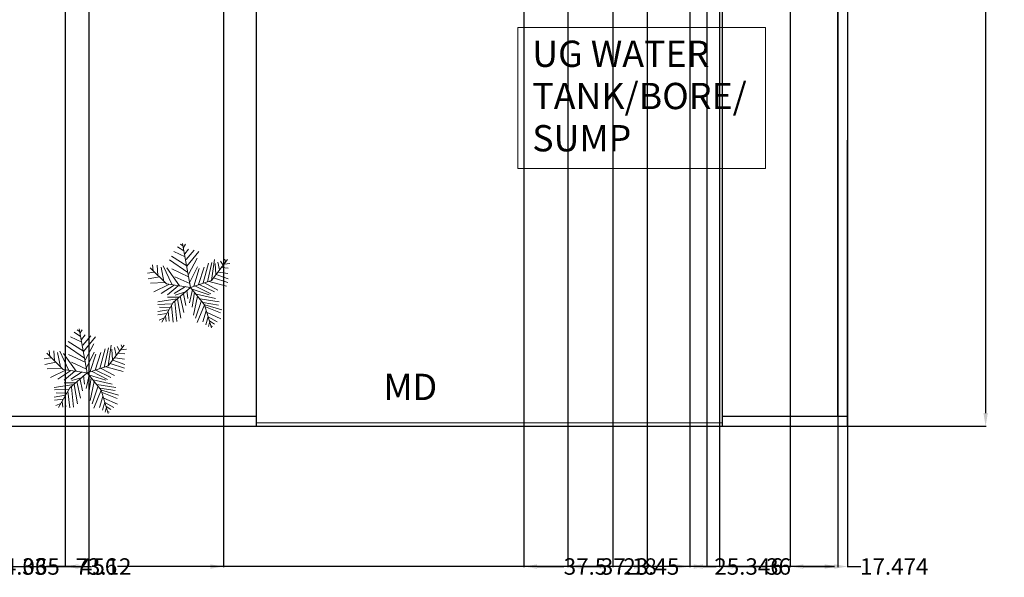
# Model space of a CAD drawing. Units: inches. Extents: x 460 to 1030, y -658 to 271.
# Tile 4 of 10: x 728 to 1028, y -658 to -488. Entities that reach past the tile are written whole.
import ezdxf

# ---------------------------------------------------------------- set-up
doc = ezdxf.new("R2010")
doc.units = ezdxf.units.IN
doc.header["$MEASUREMENT"] = 0
for name, color, linetype, lineweight in [('A-ANNO-DIMS', 2, 'Continuous', 18), ('A-ANNO-TEXT', 7, 'Continuous', 18), ('C-ANNO-TEXT', 7, 'Continuous', 18), ('C-PROP', 7, 'Continuous', 25), ('C-SITE-GATE', 3, 'Continuous', 18), ('C-UTIL', 8, 'Continuous', 18), ('L-PLNT', 94, 'Continuous', 13)]:
    doc.layers.add(name, color=color, linetype=linetype, lineweight=lineweight)
doc.styles.get("Standard").update_dxf_attribs({"font": 'arial.ttf'})
doc.dimstyles.get("Standard").update_dxf_attribs({"dimtxt": 5, "dimasz": 4, "dimexe": 0.18, "dimexo": 0.0625, "dimgap": 0.09, "dimtad": 0, "dimtih": 1, "dimtoh": 1, "dimdec": 1, "dimzin": 0, "dimdsep": 46, "dimlunit": 4, "dimtxsty": 'Standard', "dimcen": 0.09, "dimadec": 0, "dimazin": 0, "dimtfac": 1, "dimtdec": 1, "dimtofl": 0, "dimtmove": 0, "dimatfit": 3, "dimfxl": 1, "dimtolj": 1, "dimtzin": 0, "dimarcsym": 0})

# ---------------------------------------------------------------- blocks, each defined once
blk = doc.blocks.new('*U11')
for p, q in [((-221.9198, 1197.3052), (-433.5526, 1338.8594)), ((-258.7244, 1362.456), (-332.3336, 1421.4348)), ((0, 0), (-266.7, 1447.8)), ((-231.1146, 1315.2628), (-166.7002, 1421.4348)), ((-129.8956, 713.6638), (-626.7704, 1032.1544)), ((-185.1152, 1008.5578), (-553.1612, 1185.4942)), ((-194.31, 1102.9442), (-65.4812, 1256.284)), ((-148.3106, 914.1968), (118.5418, 1220.9018)), ((-129.8956, 701.8528), (265.7602, 1185.4942)), ((-1234.059, 536.7274), (-1252.4486, 737.2604)), ((-1105.2302, 725.4494), (-1077.6458, 395.1732)), ((-976.4268, 666.4706), (-884.4026, 194.6402)), ((-902.8176, 713.6638), (-617.5756, 100.2538)), ((-93.091, 489.5342), (-700.3796, 902.3858)), ((-74.7014, 418.7444), (219.7608, 961.39)), ((-28.6766, 171.0436), (228.9556, 678.2816)), ((256.5654, 88.4682), (449.7832, 666.4706)), ((412.9786, 147.447), (587.8068, 796.2392)), ((560.197, 182.8292), (698.2206, 819.8358)), ((685.8, 228.6), (1219.2, 914.4)), ((689.0258, 230.0224), (790.2448, 914.1968)), ((808.6344, 784.4282), (827.0494, 418.7444)), ((891.4384, 831.6214), (946.658, 572.1096)), ((983.4626, 867.0036), (1066.2666, 725.4494)), ((1029.462, 654.685), (1241.0948, 631.0884)), ((1112.2914, 760.8316), (1296.3144, 784.4282)), ((1121.4862, 925.9824), (1149.0706, 831.6214)), ((-1206.4492, 501.3198), (-1418.082, 465.9376)), ((-1031.621, 347.98), (-1399.667, 277.1902)), ((-800.1, 114.3), (-1333.5, 647.7)), ((-369.1382, 53.086), (-783.1836, 642.874)), ((-617.5756, 607.4918), (-74.7014, 347.98)), ((-525.5514, 347.98), (-28.6766, 123.8504)), ((100.1268, 41.275), (284.1498, 619.2774)), ((845.439, 418.7444), (1241.0948, 277.1902)), ((919.0482, 501.3198), (1222.6798, 454.152)), ((-847.598, 159.2326), (-1326.0578, 135.636)), ((-718.7946, 88.4682), (-1215.644, -147.447)), ((-543.9664, 76.6572), (-967.2066, -206.4512)), ((0, 0), (-800.1, 114.3)), ((-405.9428, 53.086), (-764.794, -241.8334)), ((0, 0), (-571.5, -495.3)), ((-166.7002, 29.4894), (-543.9664, -206.4512)), ((0, 0), (685.8, 228.6)), ((0, 0), (457.2, -571.5)), ((164.5412, 41.275), (661.416, -218.2368)), ((284.1498, 88.4682), (781.0246, -147.447)), ((458.978, 147.447), (891.4384, -88.4682)), ((615.4166, 194.6402), (1185.8752, 41.275)), ((753.4148, 312.5978), (1222.6798, 159.2326)), ((-387.5278, -324.4088), (-764.794, -324.4088)), ((-166.7002, -147.447), (-507.1618, -253.619)), ((-341.5284, -289.0012), (-221.9198, -831.6214)), ((-240.3094, -218.2368), (-157.5054, -595.7062)), ((-120.7008, -88.4682), (-93.091, -371.5766)), ((63.3222, -76.6826), (-37.8714, -513.1308)), ((44.9326, -64.897), (615.4166, -241.8334)), ((127.7366, -159.258), (54.1274, -654.685)), ((228.9556, -289.0012), (90.932, -914.1968)), ((192.151, -230.0224), (817.8292, -371.5766)), ((-442.7474, -383.3876), (-1086.8406, -477.7486)), ((-617.5756, -548.5384), (-1077.6458, -560.324)), ((-571.5, -495.3), (-952.5, -1143)), ((-635.9652, -607.5172), (-580.771, -1150.1374)), ((-525.5514, -465.963), (-451.9422, -1126.5408)), ((-433.5526, -383.3876), (-323.1134, -1020.3688)), ((357.759, -430.5554), (164.5412, -1020.3688)), ((458.978, -572.1096), (210.5406, -1161.923)), ((311.7596, -383.3876), (937.4378, -477.7486)), ((412.9786, -501.3452), (919.0482, -583.9206)), ((457.2, -571.5), (685.8, -1333.5)), ((468.1982, -572.1096), (1029.462, -737.2604)), ((486.5878, -642.8994), (983.4626, -843.4324)), ((-718.7946, -737.2604), (-1086.8406, -796.2392)), ((-783.1836, -867.029), (-1077.6458, -902.4112)), ((-681.9646, -666.496), (-1022.4262, -654.685)), ((-829.2084, -937.7934), (-810.7934, -1126.5408)), ((-737.1842, -784.4536), (-709.5744, -1114.7298)), ((514.1976, -772.6426), (403.7838, -1138.3264)), ((578.612, -961.39), (495.7826, -1232.7128)), ((541.8074, -831.6214), (992.6574, -1032.1544)), ((578.612, -973.1756), (873.0488, -1138.3264)), ((-875.2078, -1008.5832), (-1040.8412, -1079.3476)), ((624.6114, -1161.923), (587.8068, -1291.6916)), ((624.6114, -1102.9442), (781.0246, -1209.1162)), ((679.8056, -1268.095), (716.6102, -1291.6916))]:
    blk.add_line(p, q)
blk = doc.blocks.new('*D39')
at = {"layer": 'A-ANNO-DIMS', "color": 0, "lineweight": -2, "transparency": 16777216}
for p, q in [((523.8, -611.79), (523.8, -654.61)), ((979.8, -611.79), (979.8, -654.61)), ((527.8, -654.43), (746.08, -654.43)), ((975.8, -654.43), (757.51, -654.43))]:
    blk.add_line(p, q, dxfattribs=at)
at = {"layer": 'A-ANNO-DIMS', "color": 0, "transparency": 16777216}
for points in [[(527.8, -653.77), (527.8, -655.1), (523.8, -654.43)], [(975.8, -653.77), (975.8, -655.1), (979.8, -654.43)]]:
    blk.add_solid(points, dxfattribs=at)
at = {"layer": 'Defpoints', "color": 0, "transparency": 16777216}
for p in [(523.8, -611.73), (979.8, -611.73), (979.8, -654.43)]:
    blk.add_point(p, dxfattribs=at)
at = {"layer": 'A-ANNO-DIMS', "color": 0, "transparency": 16777216, "insert": (751.8, -654.43), "char_height": 5, "attachment_point": 5}
blk.add_mtext('\\A1;456', dxfattribs=at)
blk = doc.blocks.new('*D42')
at = {"layer": 'A-ANNO-DIMS', "color": 0, "lineweight": -2, "transparency": 16777216}
for p, q in [((940.86, -287.73), (1022.03, -287.73)), ((1021.85, -291.73), (1021.85, -447.08)), ((1021.85, -607.73), (1021.85, -452.37)), ((979.86, -611.73), (1022.03, -611.73))]:
    blk.add_line(p, q, dxfattribs=at)
at = {"layer": 'A-ANNO-DIMS', "color": 0, "transparency": 16777216}
for points in [[(1021.18, -291.73), (1022.51, -291.73), (1021.85, -287.73)], [(1021.18, -607.73), (1022.51, -607.73), (1021.85, -611.73)]]:
    blk.add_solid(points, dxfattribs=at)
at = {"layer": 'Defpoints', "color": 0, "transparency": 16777216}
for p in [(940.8, -287.73), (1021.85, -287.73), (979.8, -611.73)]:
    blk.add_point(p, dxfattribs=at)
at = {"layer": 'A-ANNO-DIMS', "color": 0, "transparency": 16777216, "insert": (1021.85, -449.73), "char_height": 5, "attachment_point": 5}
blk.add_mtext('\\A1;324', dxfattribs=at)
blk = doc.blocks.new('*D45')
at = {"layer": 'A-ANNO-DIMS', "color": 0, "lineweight": -2, "transparency": 16777216}
for p, q in [((976.8, 126.21), (976.8, -654.61)), ((940.8, 90.21), (940.8, -654.61)), ((944.8, -654.43), (955.13, -654.43)), ((972.8, -654.43), (962.46, -654.43))]:
    blk.add_line(p, q, dxfattribs=at)
at = {"layer": 'A-ANNO-DIMS', "color": 0, "transparency": 16777216}
for points in [[(944.8, -653.77), (944.8, -655.1), (940.8, -654.43)], [(972.8, -653.77), (972.8, -655.1), (976.8, -654.43)]]:
    blk.add_solid(points, dxfattribs=at)
at = {"layer": 'Defpoints', "color": 0, "transparency": 16777216}
for p in [(976.8, 126.27), (940.8, 90.27), (976.8, -654.43)]:
    blk.add_point(p, dxfattribs=at)
at = {"layer": 'A-ANNO-DIMS', "color": 0, "transparency": 16777216, "insert": (958.8, -654.43), "char_height": 5, "attachment_point": 5}
blk.add_mtext('\\A1;36', dxfattribs=at)
blk = doc.blocks.new('*D46')
at = {"layer": 'A-ANNO-DIMS', "color": 0, "lineweight": -2, "transparency": 16777216}
for p, q in [((936.98, 127.21), (936.98, -654.61)), ((962.32, 127.21), (962.32, -654.61)), ((932.98, -654.43), (928.98, -654.43)), ((966.32, -654.43), (970.32, -654.43))]:
    blk.add_line(p, q, dxfattribs=at)
at = {"layer": 'A-ANNO-DIMS', "color": 0, "transparency": 16777216}
for points in [[(932.98, -653.77), (932.98, -655.1), (936.98, -654.43)], [(966.32, -653.77), (966.32, -655.1), (962.32, -654.43)]]:
    blk.add_solid(points, dxfattribs=at)
at = {"layer": 'Defpoints', "color": 0, "transparency": 16777216}
for p in [(936.98, 127.27), (962.32, 127.27), (962.32, -654.43)]:
    blk.add_point(p, dxfattribs=at)
at = {"layer": 'A-ANNO-DIMS', "color": 0, "transparency": 16777216, "insert": (949.65, -654.43), "char_height": 5, "attachment_point": 5}
blk.add_mtext('\\A1;25.346', dxfattribs=at)
blk = doc.blocks.new('*D47')
at = {"layer": 'A-ANNO-DIMS', "color": 0, "lineweight": -2, "transparency": 16777216}
for p, q in [((962.32, 129.21), (962.32, -654.61)), ((979.8, 129.21), (979.8, -654.61)), ((966.32, -654.43), (975.8, -654.43)), ((979.8, -654.43), (983.8, -654.43))]:
    blk.add_line(p, q, dxfattribs=at)
at = {"layer": 'A-ANNO-DIMS', "color": 0, "transparency": 16777216}
for points in [[(966.32, -653.77), (966.32, -655.1), (962.32, -654.43)], [(975.8, -653.77), (975.8, -655.1), (979.8, -654.43)]]:
    blk.add_solid(points, dxfattribs=at)
at = {"layer": 'Defpoints', "color": 0, "transparency": 16777216}
for p in [(962.32, 129.27), (979.8, 129.27), (979.8, -654.43)]:
    blk.add_point(p, dxfattribs=at)
at = {"layer": 'A-ANNO-DIMS', "color": 0, "transparency": 16777216, "insert": (994.02, -654.43), "char_height": 5, "attachment_point": 5}
blk.add_mtext('\\A1;17.474', dxfattribs=at)
blk = doc.blocks.new('*D48')
at = {"layer": 'A-ANNO-DIMS', "color": 0, "lineweight": -2, "transparency": 16777216}
for p, q in [((799.88, -611.66), (799.88, 267.89)), ((803.88, 267.71), (860.58, 267.71)), ((937.7, 267.71), (881, 267.71)), ((941.7, -611.66), (941.7, 267.89))]:
    blk.add_line(p, q, dxfattribs=at)
at = {"layer": 'A-ANNO-DIMS', "color": 0, "transparency": 16777216}
for points in [[(803.88, 268.38), (803.88, 267.04), (799.88, 267.71)], [(937.7, 268.38), (937.7, 267.04), (941.7, 267.71)]]:
    blk.add_solid(points, dxfattribs=at)
at = {"layer": 'Defpoints', "color": 0, "transparency": 16777216}
for p in [(941.7, 267.71), (799.88, -611.73), (941.7, -611.73)]:
    blk.add_point(p, dxfattribs=at)
at = {"layer": 'A-ANNO-DIMS', "color": 0, "transparency": 16777216, "insert": (870.79, 267.71), "char_height": 5, "attachment_point": 5}
blk.add_mtext('\\A1;141.82', dxfattribs=at)
blk = doc.blocks.new('*D49')
at = {"layer": 'A-ANNO-DIMS', "color": 0, "lineweight": -2, "transparency": 16777216}
for p, q in [((941.7, -608.66), (941.7, 267.89)), ((945.7, 267.71), (953.15, 267.71)), ((972.8, 267.71), (965.35, 267.71)), ((976.8, -608.66), (976.8, 267.89))]:
    blk.add_line(p, q, dxfattribs=at)
at = {"layer": 'A-ANNO-DIMS', "color": 0, "transparency": 16777216}
for points in [[(945.7, 268.38), (945.7, 267.04), (941.7, 267.71)], [(972.8, 268.38), (972.8, 267.04), (976.8, 267.71)]]:
    blk.add_solid(points, dxfattribs=at)
at = {"layer": 'Defpoints', "color": 0, "transparency": 16777216}
for p in [(976.8, 267.71), (941.7, -608.73), (976.8, -608.73)]:
    blk.add_point(p, dxfattribs=at)
at = {"layer": 'A-ANNO-DIMS', "color": 0, "transparency": 16777216, "insert": (959.25, 267.71), "char_height": 5, "attachment_point": 5}
blk.add_mtext('\\A1;35.1', dxfattribs=at)
blk = doc.blocks.new('*D53')
at = {"layer": 'A-ANNO-DIMS', "color": 0, "lineweight": -2, "transparency": 16777216}
for p, q in [((908.35, -281.79), (908.35, -654.61)), ((931.8, -281.79), (931.8, -654.61)), ((904.35, -654.43), (900.35, -654.43)), ((935.8, -654.43), (939.8, -654.43))]:
    blk.add_line(p, q, dxfattribs=at)
at = {"layer": 'A-ANNO-DIMS', "color": 0, "transparency": 16777216}
for points in [[(904.35, -653.77), (904.35, -655.1), (908.35, -654.43)], [(935.8, -653.77), (935.8, -655.1), (931.8, -654.43)]]:
    blk.add_solid(points, dxfattribs=at)
at = {"layer": 'Defpoints', "color": 0, "transparency": 16777216}
for p in [(908.35, -281.73), (931.8, -281.73), (931.8, -654.43)]:
    blk.add_point(p, dxfattribs=at)
at = {"layer": 'A-ANNO-DIMS', "color": 0, "transparency": 16777216, "insert": (920.07, -654.43), "char_height": 5, "attachment_point": 5}
blk.add_mtext('\\A1;23.45', dxfattribs=at)
blk = doc.blocks.new('*D54')
at = {"layer": 'A-ANNO-DIMS', "color": 0, "lineweight": -2, "transparency": 16777216}
for p, q in [((894.61, -141.78), (894.61, -654.61)), ((931.8, -141.78), (931.8, -654.61)), ((898.61, -654.43), (904.68, -654.43)), ((927.8, -654.43), (921.73, -654.43))]:
    blk.add_line(p, q, dxfattribs=at)
at = {"layer": 'A-ANNO-DIMS', "color": 0, "transparency": 16777216}
for points in [[(898.61, -653.77), (898.61, -655.1), (894.61, -654.43)], [(927.8, -653.77), (927.8, -655.1), (931.8, -654.43)]]:
    blk.add_solid(points, dxfattribs=at)
at = {"layer": 'Defpoints', "color": 0, "transparency": 16777216}
for p in [(894.61, -141.72), (931.8, -141.72), (931.8, -654.43)]:
    blk.add_point(p, dxfattribs=at)
at = {"layer": 'A-ANNO-DIMS', "color": 0, "transparency": 16777216, "insert": (913.2, -654.43), "char_height": 5, "attachment_point": 5}
blk.add_mtext('\\A1;37.18', dxfattribs=at)
blk = doc.blocks.new('*D57')
at = {"layer": 'A-ANNO-DIMS', "color": 0, "lineweight": -2, "transparency": 16777216}
for p, q in [((717.53, -38.79), (717.53, -654.61)), ((741.59, -38.79), (741.59, -654.61)), ((713.53, -654.43), (709.53, -654.43)), ((745.59, -654.43), (749.59, -654.43))]:
    blk.add_line(p, q, dxfattribs=at)
at = {"layer": 'A-ANNO-DIMS', "color": 0, "transparency": 16777216}
for points in [[(713.53, -653.77), (713.53, -655.1), (717.53, -654.43)], [(745.59, -653.77), (745.59, -655.1), (741.59, -654.43)]]:
    blk.add_solid(points, dxfattribs=at)
at = {"layer": 'Defpoints', "color": 0, "transparency": 16777216}
for p in [(717.53, -38.73), (741.59, -38.73), (741.59, -654.43)]:
    blk.add_point(p, dxfattribs=at)
at = {"layer": 'A-ANNO-DIMS', "color": 0, "transparency": 16777216, "insert": (729.56, -654.43), "char_height": 5, "attachment_point": 5}
blk.add_mtext('\\A1;24.065', dxfattribs=at)
blk = doc.blocks.new('*D69')
at = {"layer": 'A-ANNO-DIMS', "color": 0, "lineweight": -2, "transparency": 16777216}
for p, q in [((881.27, 90.21), (881.27, -654.61)), ((918.77, 90.21), (918.77, -654.61)), ((885.27, -654.43), (893.42, -654.43)), ((914.77, -654.43), (906.62, -654.43))]:
    blk.add_line(p, q, dxfattribs=at)
at = {"layer": 'A-ANNO-DIMS', "color": 0, "transparency": 16777216}
for points in [[(885.27, -653.77), (885.27, -655.1), (881.27, -654.43)], [(914.77, -653.77), (914.77, -655.1), (918.77, -654.43)]]:
    blk.add_solid(points, dxfattribs=at)
at = {"layer": 'Defpoints', "color": 0, "transparency": 16777216}
for p in [(881.27, 90.27), (918.77, 90.27), (918.77, -654.43)]:
    blk.add_point(p, dxfattribs=at)
at = {"layer": 'A-ANNO-DIMS', "color": 0, "transparency": 16777216, "insert": (900.02, -654.43), "char_height": 5, "attachment_point": 5}
blk.add_mtext('\\A1;37.5', dxfattribs=at)
blk = doc.blocks.new('*D70')
at = {"layer": 'A-ANNO-DIMS', "color": 0, "lineweight": -2, "transparency": 16777216}
for p, q in [((716.71, -287.79), (716.71, -654.61)), ((789.82, -287.79), (789.82, -654.61)), ((720.71, -654.43), (744.79, -654.43)), ((785.82, -654.43), (761.75, -654.43))]:
    blk.add_line(p, q, dxfattribs=at)
at = {"layer": 'A-ANNO-DIMS', "color": 0, "transparency": 16777216}
for points in [[(720.71, -653.77), (720.71, -655.1), (716.71, -654.43)], [(785.82, -653.77), (785.82, -655.1), (789.82, -654.43)]]:
    blk.add_solid(points, dxfattribs=at)
at = {"layer": 'Defpoints', "color": 0, "transparency": 16777216}
for p in [(716.71, -287.73), (789.82, -287.73), (789.82, -654.43)]:
    blk.add_point(p, dxfattribs=at)
at = {"layer": 'A-ANNO-DIMS', "color": 0, "transparency": 16777216, "insert": (753.27, -654.43), "char_height": 5, "attachment_point": 5}
blk.add_mtext('\\A1;73.12', dxfattribs=at)
blk = doc.blocks.new('*D72')
at = {"layer": 'A-ANNO-DIMS', "color": 0, "lineweight": -2, "transparency": 16777216}
for p, q in [((715.8, 68.25), (715.8, -654.61)), ((748.8, 57.75), (748.8, -654.61)), ((719.8, -654.43), (728.63, -654.43)), ((744.8, -654.43), (735.97, -654.43))]:
    blk.add_line(p, q, dxfattribs=at)
at = {"layer": 'A-ANNO-DIMS', "color": 0, "transparency": 16777216}
for points in [[(719.8, -653.77), (719.8, -655.1), (715.8, -654.43)], [(744.8, -653.77), (744.8, -655.1), (748.8, -654.43)]]:
    blk.add_solid(points, dxfattribs=at)
at = {"layer": 'Defpoints', "color": 0, "transparency": 16777216}
for p in [(715.8, 68.31), (748.8, 57.81), (748.8, -654.43)]:
    blk.add_point(p, dxfattribs=at)
at = {"layer": 'A-ANNO-DIMS', "color": 0, "transparency": 16777216, "insert": (732.3, -654.43), "char_height": 5, "attachment_point": 5}
blk.add_mtext('\\A1;33', dxfattribs=at)

msp = doc.modelspace()

# ---------------------------------------------------------------- linework, layer by layer
at = {"layer": 'C-PROP'}
for p, q in [((979.7961, 129.2738), (979.7961, -524.7262)), ((976.7961, -485.7262), (976.7961, -608.7262)), ((979.7961, -611.7262), (979.7961, -524.7262)), ((526.7961, -608.7262), (799.8801, -608.7262)), ((941.6978, -608.7262), (979.7961, -608.7262)), ((523.7961, -611.7262), (979.7961, -611.7262))]:
    msp.add_line(p, q, dxfattribs=at)
at = {"layer": 'C-SITE-GATE'}
for p, q in [((799.8801, -608.7262), (799.8801, -611.7262)), ((799.8801, -610.7262), (941.6978, -610.7262)), ((941.6978, -611.7262), (941.6978, -608.7262)), ((799.8801, -611.7262), (941.6978, -611.7262))]:
    msp.add_line(p, q, dxfattribs=at)
at = {"layer": 'C-UTIL'}
msp.add_lwpolyline([(879.4207, -490.3806), (954.8498, -490.3806), (954.8498, -533.3441), (879.4207, -533.3441)], close=True, dxfattribs=at)

# ---------------------------------------------------------------- block references
at = {"layer": 'L-PLNT', "xscale": 0.0092368434635362, "yscale": 0.0092368434635362, "zscale": 0.0092368434635362}
for p in [(779.8219, -569.4876), (748.3571, -595.5181)]:
    msp.add_blockref('*U11', p, dxfattribs=at)

# ---------------------------------------------------------------- texts
at = {"layer": 'A-ANNO-TEXT'}
msp.add_text('MD', height=8, dxfattribs=at).set_placement((838.51, -603.7857))
at = {"layer": 'C-ANNO-TEXT'}
for s, p in [('UG WATER', (883.8097, -502.4182)), ('TANK/BORE/', (883.8097, -515.2695)), ('SUMP', (883.8097, -528.1207))]:
    msp.add_text(s, height=8, dxfattribs=at).set_placement(p)

# ---------------------------------------------------------------- dimensions: what is measured, and where the dimension line sits
at = {"layer": 'A-ANNO-DIMS'}
for base, p1, p2, override, picture, middle in [((941.6978, 267.7108), (799.8801, -611.7262), (941.6978, -611.7262), {"dimdec": 2, "dimlfac": 1, "dimrnd": 0, "dimzin": 0, "dimdsep": 46, "dimlunit": 2}, '*D48', (870.7889, 267.7108)), ((976.7961, 267.7108), (941.6978, -608.7262), (976.7961, -608.7262), {"dimdec": 1, "dimlfac": 1, "dimrnd": 0, "dimzin": 0, "dimdsep": 46, "dimlunit": 2}, '*D49', (959.247, 267.7108)), ((979.7961, -654.4339), (962.3217, 129.2738), (979.7961, 129.2738), {"dimdec": 3, "dimlfac": 1, "dimrnd": 0, "dimzin": 0, "dimdsep": 46, "dimlunit": 2}, '*D47', (994.0191, -654.4339)), ((962.3217, -654.4339), (936.9757, 127.2738), (962.3217, 127.2738), {"dimdec": 3, "dimlfac": 1, "dimrnd": 0, "dimzin": 0, "dimdsep": 46, "dimlunit": 2}, '*D46', (949.6487, -654.4339)), ((976.7961, -654.4339), (940.7961, 90.2738), (976.7961, 126.2738), {"dimdec": 0, "dimlfac": 1, "dimrnd": 0, "dimzin": 0, "dimdsep": 46, "dimlunit": 2}, '*D45', (958.7961, -654.4339)), ((918.7723, -654.4339), (881.2728, 90.2738), (918.7723, 90.2738), {"dimdec": 1, "dimlfac": 1, "dimrnd": 0, "dimzin": 0, "dimdsep": 46, "dimlunit": 2}, '*D69', (900.0226, -654.4339)), ((748.7961, -654.4339), (715.7961, 68.3148), (748.7961, 57.8148), {"dimdec": 0, "dimlfac": 1, "dimrnd": 0, "dimzin": 0, "dimdsep": 46, "dimlunit": 2}, '*D72', (732.2961, -654.4339)), ((741.5908, -654.4339), (717.5258, -38.7262), (741.5908, -38.7262), {"dimdec": 3, "dimlfac": 1, "dimrnd": 0, "dimzin": 0, "dimdsep": 46, "dimlunit": 2}, '*D57', (729.5583, -654.4339)), ((931.7961, -654.4339), (894.6132, -141.7212), (931.7961, -141.7212), {"dimdec": 2, "dimlfac": 1, "dimrnd": 0, "dimzin": 0, "dimdsep": 46, "dimlunit": 2}, '*D54', (913.2047, -654.4339)), ((931.7961, -654.4339), (908.3452, -281.7262), (931.7961, -281.7262), {"dimdec": 2, "dimlfac": 1, "dimrnd": 0, "dimzin": 0, "dimdsep": 46, "dimlunit": 2}, '*D53', (920.0707, -654.4339)), ((789.8237, -654.4339), (716.7073, -287.7262), (789.8237, -287.7262), {"dimdec": 2, "dimlfac": 1, "dimrnd": 0, "dimzin": 0, "dimdsep": 46, "dimlunit": 2}, '*D70', (753.2655, -654.4339)), ((979.7961, -654.4339), (523.7961, -611.7262), (979.7961, -611.7262), {"dimdec": 0, "dimlfac": 1, "dimrnd": 0, "dimzin": 0, "dimdsep": 46, "dimlunit": 2}, '*D39', (751.7961, -654.4339))]:
    dim = msp.add_linear_dim(base=base, p1=p1, p2=p2, dimstyle='Standard', override=override, dxfattribs=at)
    dim.commit()
    dim.dimension.update_dxf_attribs({"geometry": picture, "text_midpoint": middle})
dim = msp.add_linear_dim(base=(1021.8461, -287.7262), p1=(979.7961, -611.7262), p2=(940.7961, -287.7262), angle=90, dimstyle='Standard', override={"dimdec": 0, "dimlfac": 1, "dimrnd": 0, "dimzin": 0, "dimdsep": 46, "dimlunit": 2}, dxfattribs=at)
dim.commit()
dim.dimension.update_dxf_attribs({"geometry": '*D42', "text_midpoint": (1021.8461, -449.7262)})

doc.saveas('drawing.dxf')
